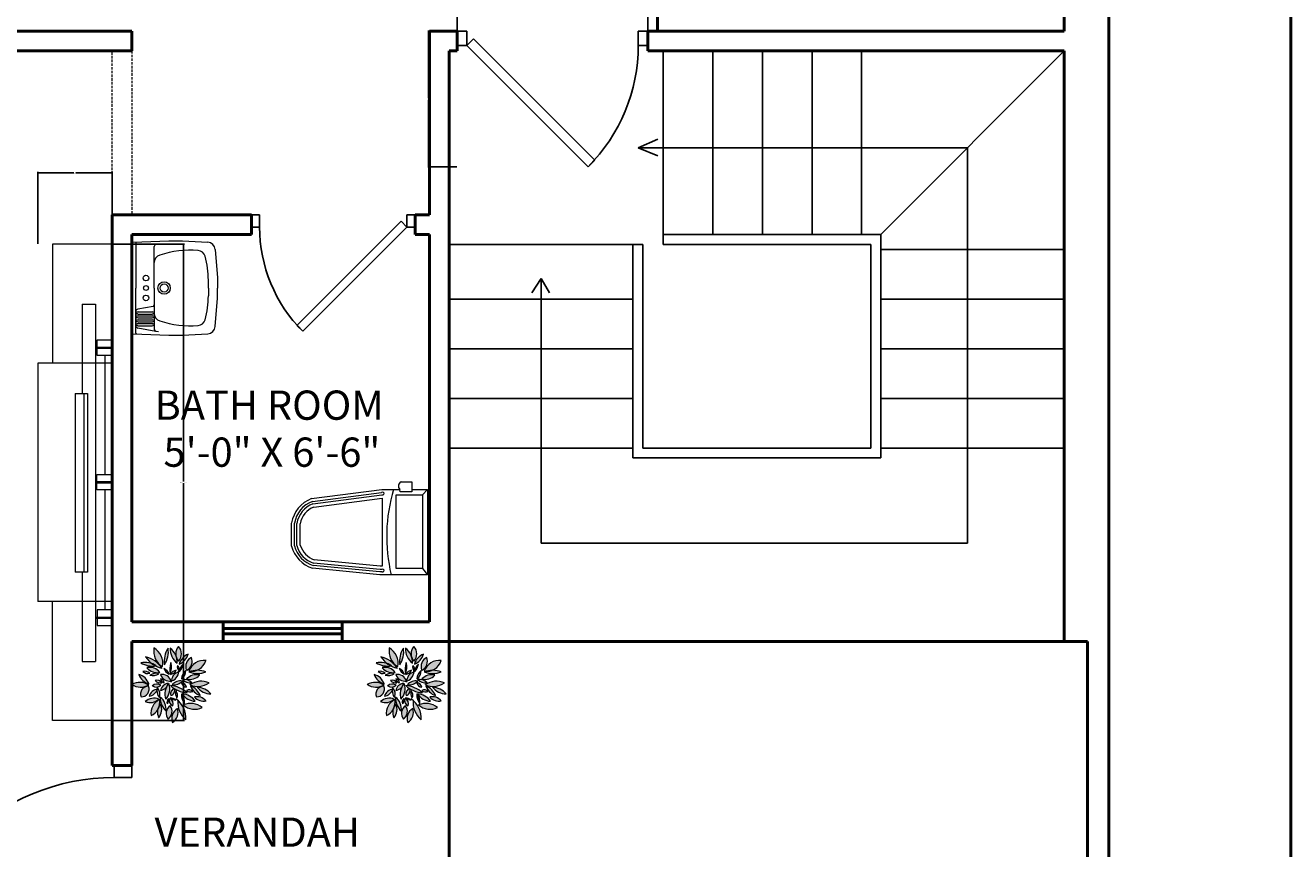
# Model space of a CAD drawing. Units: inches. Extents: x 64 to 1167, y 117 to 939.
# Tile 4 of 56: x 258 to 513, y 272 to 438. Entities that reach past the tile are written whole.
import ezdxf

# ---------------------------------------------------------------- set-up
doc = ezdxf.new("R2010")
doc.units = ezdxf.units.IN
doc.header["$MEASUREMENT"] = 0
doc.linetypes.add('DASHED', pattern=[0.75, 0.5, -0.25])
for name, color, linetype, lineweight in [('A-ANNO-DIMS', 2, 'Continuous', 18), ('A-ANNO-TEXT', 7, 'Continuous', 25), ('A-ANNO-TTLB', 7, 'Continuous', 50), ('A-DOOR', 4, 'Continuous', 25), ('A-FLOR-FIXT', 8, 'Continuous', 18), ('A-FLOR-OVHD', 8, 'DASHED', 18), ('A-FLOR-STRS', 3, 'Continuous', 25), ('A-FURN', 8, 'Continuous', 18), ('A-WALL', 7, 'Continuous', 50)]:
    doc.layers.add(name, color=color, linetype=linetype, lineweight=lineweight)
doc.styles.get("Standard").update_dxf_attribs({"font": 'arial.ttf'})
doc.dimstyles.get("Standard").update_dxf_attribs({"dimtxt": 0.18, "dimasz": 0.18, "dimexe": 0.18, "dimexo": 0.0625, "dimgap": 0.09, "dimtad": 0, "dimtih": 1, "dimtoh": 1, "dimdec": 4, "dimzin": 0, "dimdsep": 46, "dimtxsty": 'Standard', "dimcen": 0.09, "dimadec": 0, "dimazin": 0, "dimtfac": 1, "dimtdec": 4, "dimtofl": 0, "dimtmove": 0, "dimatfit": 3, "dimfxl": 1, "dimtolj": 1, "dimtzin": 0, "dimarcsym": 0})

# ---------------------------------------------------------------- blocks, each defined once
blk = doc.blocks.new('A$C68901CC0')
for p, q in [((10.95, 26.62), (12.35, 28.01)), ((12.35, 28.01), (37.4, 2.95)), ((36.01, 1.56), (10.95, 26.62)), ((0, 2.95), (0, 0)), ((1.97, 2.95), (0, 2.95)), ((1.97, 0), (1.97, 2.95)), ((37.4, 2.95), (36.01, 1.56)), ((37.4, 2.95), (37.4, 0)), ((39.37, 2.95), (37.4, 2.95)), ((39.37, 0), (39.37, 2.95)), ((0, 0), (1.97, 0)), ((37.4, 0), (39.37, 0))]:
    blk.add_line(p, q)
blk.add_arc((37.4, 2.95), 35.43, 135, 180)
blk = doc.blocks.new("CONSOLE 8'x1'3")
for p, q in [((-48, 0), (48, 0)), ((48, 0), (48, -12)), ((-48, 0), (-48, -12)), ((-24, 0), (-24, -15)), ((24, 0), (24, -15)), ((-48, -12), (-24, -12)), ((48, -12), (24, -12)), ((-24, -15), (24, -15))]:
    blk.add_line(p, q)
blk = doc.blocks.new('A$C2B992F40')
for p, q in [((39.2, 615.2), (39.2, 696.2)), ((39.2, 696.2), (475.7, 696.2)), ((66.8, 669.7), (39.2, 696.2)), ((66.8, 534.6), (66.8, 669.7)), ((66.8, 669.7), (444.2, 669.7)), ((444.2, 669.7), (475.7, 696.2)), ((444.2, 669.7), (444.2, 534.6)), ((475.7, 696.2), (475.7, 509.8)), ((0, 561.3), (0, 615.2)), ((0, 615.2), (51.5, 615.2)), ((51.5, 615.2), (51.5, 556.4)), ((51.5, 556.4), (39.2, 553.9)), ((39.2, 522.1), (39.2, 553.9)), ((40.1, 461.2), (39.2, 522.1)), ((444.2, 534.6), (66.8, 534.6)), ((86.6, 102.5), (40.1, 461.2)), ((101, 106.1), (55, 460.6)), ((112.5, 109), (66.6, 462.1)), ((84.2, 464.4), (431.5, 464.4)), ((129.7, 113.4), (84.2, 464.4)), ((431.5, 454), (399.6, 116.2)), ((431.5, 464.4), (431.5, 454)), ((449.2, 464.4), (449.2, 453.2)), ((461, 464.4), (461, 452.6)), ((475.7, 509.8), (475.7, 451.9)), ((449.2, 453.2), (417, 112.5)), ((461, 452.6), (428.6, 110.1)), ((475.7, 451.9), (443.1, 107.2)), ((330.1, 0), (211.3, 0)), ((328.2, 14.7), (212.5, 14.7)), ((326.7, 26.5), (213.4, 26.5)), ((324.2, 44.1), (215, 44.1))]:
    blk.add_line(p, q)
for centre, radius, start, end in [((22.2, 571.4), 24.4, 204.49972, 314.26101), ((280.3, 1327.8), 841, 253.34642, 283.43557), ((60.2, 466.1), 7.56, 328.52932, 226.26991), ((454.4, 466.1), 7.56, 328.52932, 226.26991), ((235.9, 157), 158.9, 200.05507, 261.07522), ((235.9, 157), 144.2, 200.68762, 260.63012), ((235.9, 157), 132.4, 201.26818, 260.22173), ((235.9, 157), 114.8, 202.30203, 259.4948), ((291.5, 153.8), 114.4, 286.5809, 340.81554), ((291.5, 153.8), 132.1, 285.42576, 341.7737), ((291.5, 153.8), 143.8, 284.77755, 342.31156), ((291.5, 153.8), 158.5, 284.07165, 342.89742)]:
    blk.add_arc(centre, radius, start, end)
blk = doc.blocks.new("FLAT TV 6'")
for p, q in [((2564.73, 835.73), (2564.73, 838.99)), ((2564.97, 835.73), (2564.97, 838.99)), ((2566.41, 837.49), (2590.37, 837.49)), ((2591.81, 835.67), (2591.81, 838.93)), ((2592.05, 835.67), (2592.05, 838.93)), ((2593.49, 837.49), (2617.69, 837.49)), ((2619.13, 835.73), (2619.13, 838.99)), ((2619.37, 835.73), (2619.37, 838.99)), ((2556.05, 835.67), (2628.05, 835.67)), ((2556.05, 832.92), (2556.05, 835.67)), ((2628.05, 832.92), (2628.05, 835.67)), ((2556.05, 832.92), (2574.05, 832.92)), ((2574.05, 831.54), (2574.05, 834.04)), ((2574.05, 834.04), (2610.05, 834.04)), ((2574.05, 833.29), (2610.05, 833.29)), ((2610.05, 834.04), (2610.05, 831.54)), ((2610.05, 832.92), (2628.05, 832.92)), ((2574.05, 831.54), (2610.05, 831.54))]:
    blk.add_line(p, q)
for points in [[(2563.29, 838.99), (2566.41, 838.99), (2566.41, 835.99), (2563.29, 835.99)], [(2590.37, 838.93), (2593.49, 838.93), (2593.49, 835.93), (2590.37, 835.93)], [(2620.82, 838.99), (2617.69, 838.99), (2617.69, 835.99), (2620.82, 835.99)]]:
    blk.add_lwpolyline(points, close=True)
blk = doc.blocks.new('A$C172C5132')
at = {"linetype": 'ByBlock'}
h = blk.add_hatch(color=256, dxfattribs=at)
h.set_gradient(color1=(15, 138, 17), color2=(46, 92, 10), tint=1, name='HEMISPHERICAL')
h.paths.add_polyline_path([(0.0849, 0.0409, 0.236282), (0.1, 0.0045, 0.236282)])
h.paths.add_polyline_path([(0.0951, 0.0322, 0.290628), (0.1303, 0.0274, 0.290628)])
h.paths.add_polyline_path([(0.0751, 0, 0.364082), (0.0843, 0.0256, 0.364082)])
h.paths.add_polyline_path([(0.0708, 0.0309, 0.428936), (0.0669, 0.0061, 0.428936)])
h.paths.add_polyline_path([(0.0526, 0.0469, 0.243055), (0.0634, 0.0209, 0.243055)])
h.paths.add_polyline_path([(0.0509, 0.0311, -0.075692), (0.0478, 0.0235, 0.164666), (0.0495, 0.0087, 0.298636), (0.053, 0.0339, 0.03785)])
h.paths.add_polyline_path([(0.0356, 0.0126, 0.152567), (0.0478, 0.0235, -0.089408), (0.0509, 0.0311, 0.1023), (0.0513, 0.0422, 0.341288)])
h.paths.add_polyline_path([(0.0248, 0.0387, 0.299202), (0.0498, 0.0428, 0.299202)])
h.paths.add_polyline_path([(0.0475, 0.0637, 0.031182), (0.0468, 0.0616, -0.006707), (0.0473, 0.0617), (0.0473, 0.0617), (0.0473, 0.0617, -0.03138), (0.0464, 0.0594, 0.214704), (0.0508, 0.0461, 0.282795)])
h.paths.add_polyline_path([(0.0643, 0.0658, 0.211659), (0.0625, 0.043, 0.281051), (0.0686, 0.0717, 0.038772), (0.0659, 0.0683, -0.044717)])
h.paths.add_polyline_path([(0.053, 0.0591, 0.203733), (0.0643, 0.0658, -0.026656), (0.0659, 0.0683, 0.062829), (0.0673, 0.0723, 0.318582)])
h.paths.add_polyline_path([(0.0695, 0.0439, 0.403257), (0.076, 0.0304, 0.403257)])
h.paths.add_polyline_path([(0.0652, 0.0343, 0.302607), (0.0678, 0.0439, 0.302607)])
h.paths.add_polyline_path([(0.0708, 0.0452, 0.20419), (0.0817, 0.0413, 0.20419)])
h.paths.add_polyline_path([(0.0817, 0.0582, 0.262138), (0.0834, 0.0452, 0.262138)])
h.paths.add_polyline_path([(0.0721, 0.05, 0.44636), (0.0791, 0.0622, 0.44636)])
h.paths.add_polyline_path([(0.0934, 0.0526, 0.247085), (0.1173, 0.0391, 0.247085)])
h.paths.add_polyline_path([(0.0712, 0.0682, 0.171467), (0.1021, 0.0548, 0.171467)])
h.paths.add_polyline_path([(0.0747, 0.07, 0.259278), (0.0934, 0.0765, 0.259278)])
h.paths.add_polyline_path([(0.0917, 0.073, 0.365639), (0.1012, 0.0652, 0.365639)])
h.paths.add_polyline_path([(0.0934, 0.0795, 0.243415), (0.1108, 0.0735, 0.243415)])
h.paths.add_polyline_path([(0.1012, 0.0591, 0.307451), (0.1129, 0.0574, 0.307451)])
h.paths.add_polyline_path([(0.1086, 0.0674, 0.209633), (0.1264, 0.0496, 0.209633)])
h.paths.add_polyline_path([(0.1208, 0.0652, 0.21311), (0.1464, 0.0526, 0.21311)])
h.paths.add_polyline_path([(0.116, 0.0469, 0.265719), (0.1373, 0.04, 0.265719)])
h.paths.add_polyline_path([(0.1012, 0.0804, 0.271534), (0.1255, 0.0874, 0.271534)])
h.paths.add_polyline_path([(0.1204, 0.0965, -0.10541), (0.1084, 0.0945, 0.018052), (0.1055, 0.0935, 0.194763), (0.1373, 0.0935, 0.102488)])
h.paths.add_polyline_path([(0.1055, 0.0948, 0.024701), (0.1084, 0.0945, -0.072299), (0.1204, 0.0965, 0.220444), (0.1373, 0.1143, 0.361284)])
h.paths.add_polyline_path([(0.0921, 0.0808, 0.244188), (0.0999, 0.0961, 0.244188)])
h.paths.add_polyline_path([(0.0873, 0.1078, 0.236039), (0.1042, 0.1265, 0.236039)])
h.paths.add_polyline_path([(0.0843, 0.1056, 0.271887), (0.0875, 0.0951, 0.271887)])
h.paths.add_polyline_path([(0.073, 0.0766, -0.001193), (0.073, 0.0765, 0.325344), (0.0864, 0.0931, 0.324468)])
h.paths.add_polyline_path([(0.0713, 0.0905, 0.143951), (0.0721, 0.1108, 0.143951)])
h.paths.add_polyline_path([(0.0591, 0.1, 0.207976), (0.0691, 0.0891, 0.207976)])
h.paths.add_polyline_path([(0.0604, 0.1065, 0.190107), (0.0669, 0.1374, 0.190107)])
h.paths.add_polyline_path([(0.0708, 0.1374, 0.252904), (0.0838, 0.1095, 0.067921), (0.0831, 0.1182, -0.074796), (0.0813, 0.124, 0.134159)])
h.paths.add_polyline_path([(0.0813, 0.124, -0.046564), (0.0831, 0.1182, 0.072445), (0.0864, 0.1134, 0.391074), (0.0864, 0.1408, 0.229731)])
h = blk.add_hatch(color=256, dxfattribs=at)
h.set_gradient(color1=(12, 110, 14), color2=(39, 78, 9), tint=1, name='HEMISPHERICAL')
h.paths.add_polyline_path([(0.0278, 0.1013, 0.287265), (0.0517, 0.0926, 0.287265)])
h.paths.add_polyline_path([(0.0334, 0.0874, 0.245454), (0.05, 0.09, 0.245454)])
h.paths.add_polyline_path([(0.053, 0.0887, 0.362884), (0.0729, 0.0765, -0.000877), (0.073, 0.0766, 0.362272)])
h.paths.add_polyline_path([(0.053, 0.0808, 0.33327), (0.0599, 0.073, 0.33327)])
h.paths.add_polyline_path([(0.043, 0.0778, 0.302945), (0.0552, 0.0735, 0.302945)])
h.paths.add_polyline_path([(0.0378, 0.0674, 0.378763), (0.0534, 0.0687, 0.378763)])
h.paths.add_polyline_path([(0.0317, 0.0482, 0.247698), (0.0464, 0.0594, -0.032946), (0.0468, 0.0616, 0.274039)])
h.paths.add_polyline_path([(0.0169, 0.0474, 0.549808), (0.0308, 0.0669, 0.549808)])
h.paths.add_polyline_path([(0, 0.0704, 0.297781), (0.0304, 0.069, 0.297781)])
h.paths.add_polyline_path([(0.013, 0.0887, 0.248111), (0.0313, 0.0713, 0.248111)])
h.paths.add_polyline_path([(0.0204, 0.0943, 0.290415), (0.033, 0.0908, 0.290415)])
h.paths.add_polyline_path([(0.0165, 0.1104, 0.175406), (0.0437, 0.1045, -0.037323), (0.0372, 0.1086, 0.129374)])
h.paths.add_polyline_path([(0.0252, 0.1213, 0.085647), (0.0372, 0.1086, -0.054384), (0.0452, 0.1048), (0.0452, 0.1048, -0.009351), (0.0437, 0.1045, 0.060507), (0.0552, 0.1), (0.0556, 0.1006, 0.185254)])
h.paths.add_polyline_path([(0.0408, 0.1378, 0.313266), (0.0566, 0.1033), (0.0567, 0.1033, 0.313266)])
h.paths.add_polyline_path([(0.0712, 0.0891), (0.0716, 0.0886, 0.230232), (0.0821, 0.0965, 0.230232)])
h.paths.add_polyline_path([(0.0877, 0.0943), (0.0881, 0.0941, 0.179345), (0.0947, 0.1078, 0.179345)])
h.paths.add_polyline_path([(0.1008, 0.0968), (0.1016, 0.0965, 0.378282), (0.1103, 0.1204, 0.378282)])
h = blk.add_hatch(color=256, dxfattribs=at)
h.set_gradient(color1=(12, 110, 14), color2=(39, 78, 9), tint=1, name='HEMISPHERICAL')
h.paths.add_polyline_path([(0.1077, 0.0699), (0.1077, 0.0695, 0.262244), (0.1429, 0.073, 0.262244)])
h = blk.add_hatch(color=256)
h.set_gradient(color1=(12, 110, 14), color2=(39, 78, 9), tint=1, name='HEMISPHERICAL')
h.paths.add_polyline_path([(0.0925, 0.0526), (0.092, 0.0525, 0.192472), (0.0973, 0.0343, 0.192472)])
for p, q in [((0.0552, 0.1), (0.0556, 0.1006)), ((0.0566, 0.1033), (0.0567, 0.1033)), ((0.0881, 0.0941), (0.0877, 0.0943)), ((0.1016, 0.0965), (0.1008, 0.0968)), ((0.0716, 0.0886), (0.0712, 0.0891)), ((0.0925, 0.0526), (0.092, 0.0525)), ((0.1077, 0.0695), (0.1077, 0.0699))]:
    blk.add_line(p, q, dxfattribs=at)
for centre, radius, start, end in [((0.1013, 0.1271), 0.0202, 137.2816, 222.7184), ((0.0716, 0.1271), 0.0202, 317.2816, 42.7184), ((0.0135, 0.0713), 0.0513, 34.8518, 76.8329), ((0.0679, 0.1498), 0.0513, 213.7346, 255.7157), ((0.0736, 0.1319), 0.0333, 169.7437, 239.3198), ((0.024, 0.1091), 0.0333, 349.9797, 59.5558), ((0.1028, 0.1137), 0.043, 146.5506, 189.6063), ((0.0245, 0.1302), 0.043, 326.5506, 9.6063), ((0.1031, 0.1355), 0.0323, 176.7146, 233.4855), ((0.0516, 0.1114), 0.0323, 356.7146, 53.4855), ((0.1145, 0.1002), 0.0282, 111.2499, 164.3738), ((0.0771, 0.1341), 0.0282, 291.2499, 344.3738), ((0.1189, 0.1032), 0.0192, 116.5049, 199.3878), ((0.0924, 0.1134), 0.0192, 298.5878, 21.4707), ((0.0235, 0.0702), 0.0408, 57.8807, 99.8189), ((0.0382, 0.145), 0.0408, 237.8807, 279.8189), ((0.024, 0.0827), 0.0122, 42.1798, 106.9561), ((0.0295, 0.1025), 0.0122, 222.1798, 286.9561), ((0.0328, 0.0779), 0.024, 37.9495, 102.0596), ((0.0467, 0.116), 0.024, 217.9495, 282.0596), ((0.0516, 0.083), 0.0185, 19.0975, 66.0922), ((0.0766, 0.106), 0.0185, 199.0975, 246.0922), ((0.1064, 0.0993), 0.0362, 161.3279, 196.3785), ((0.037, 0.102), 0.0362, 339.0434, 14.094), ((0.0682, 0.094), 0.0182, 278.3256, 1.7816), ((0.0843, 0.0816), 0.015, 98.3028, 150.1644), ((0.0688, 0.1034), 0.015, 280.7404, 332.602), ((0.0949, 0.1031), 0.0109, 166.6712, 231.5788), ((0.0769, 0.0976), 0.0109, 342.6051, 47.5126), ((0.1094, 0.0917), 0.0218, 132.3809, 173.0513), ((0.073, 0.1098), 0.0218, 313.9894, 354.6599), ((0.0813, 0.096), 0.0186, 305.3547, 0.2444), ((0.1106, 0.0809), 0.0186, 125.3547, 180.2444), ((0.1332, 0.0855), 0.0291, 81.9405, 161.3964), ((0.1096, 0.1236), 0.0291, 261.9405, 341.3964), ((0.1214, 0.0543), 0.0422, 67.9577, 112.0423), ((0.0141, 0.0464), 0.0278, 52.0955, 120.5238), ((0.0163, 0.093), 0.0278, 234.1936, 302.622), ((0.0386, 0.0972), 0.027, 198.5093, 254.2466), ((0.0057, 0.0627), 0.027, 18.5093, 74.2466), ((0.0442, 0.0729), 0.018, 71.397, 126.5601), ((0.0392, 0.1045), 0.018, 251.397, 306.5601), ((0.0463, 0.0592), 0.0118, 53.2772, 136.2565), ((0.0458, 0.0665), 0.0116, 36.6262, 104.0418), ((0.0523, 0.0847), 0.0116, 216.6262, 284.0418), ((0.0557, 0.0706), 0.0182, 18.7265, 98.5819), ((0.0703, 0.0945), 0.0182, 198.7265, 278.5819), ((0.0512, 0.0723), 0.00872, 4.751, 78.4779), ((0.0617, 0.0816), 0.00872, 184.751, 258.4779), ((0.0508, 0.0758), 0.0168, 277.3883, 349.0703), ((0.0694, 0.0556), 0.0168, 96.3902, 168.0722), ((0.0891, 0.0524), 0.0281, 136.6356, 199.4278), ((0.0421, 0.0624), 0.0281, 316.6356, 19.4278), ((0.0911, 0.0756), 0.0182, 100.5964, 184.0524), ((0.0899, 0.0564), 0.0204, 80.1717, 138.3136), ((0.0782, 0.09), 0.0204, 260.1717, 318.3136), ((0.0918, 0.0634), 0.00957, 10.523, 90.8605), ((0.1011, 0.0748), 0.00957, 190.523, 270.8605), ((0.0962, 0.0597), 0.02, 43.3367, 98.0592), ((0.108, 0.0933), 0.02, 223.3367, 278.0592), ((0.1193, 0.0631), 0.025, 75.5726, 136.3385), ((0.1074, 0.1046), 0.025, 255.5726, 316.3385), ((0.1214, 0.1326), 0.0422, 247.9577, 292.0423), ((0.1281, 0.0402), 0.036, 65.6693, 124.4476), ((0.1222, 0.1025), 0.036, 246.2552, 305.0335), ((0.0301, 0.0527), 0.0142, 86.9965, 202.2058), ((0.0177, 0.0616), 0.0142, 266.9965, 22.2058), ((0.0285, 0.0678), 0.0198, 279.3324, 342.1699), ((0.0506, 0.0422), 0.0198, 99.3324, 162.1699), ((0.0449, 0.0769), 0.0118, 233.2772, 316.2565), ((0.0634, 0.0576), 0.0171, 157.7122, 222.4235), ((0.0348, 0.0521), 0.0171, 339.261, 43.9723), ((0.0832, 0.0444), 0.0308, 175.2839, 229.9285), ((0.0327, 0.0234), 0.0308, 355.2839, 49.9285), ((0.1057, 0.1051), 0.0505, 226.9394, 265.8583), ((0.0676, 0.0179), 0.0505, 46.9394, 85.8583), ((0.081, 0.053), 0.00941, 102.1635, 198.3798), ((0.0701, 0.0592), 0.00941, 282.1635, 18.3798), ((0.0941, 0.0533), 0.0134, 158.2119, 216.9673), ((0.0709, 0.0502), 0.0134, 338.2119, 36.9673), ((0.1173, 0.05), 0.0254, 174.4977, 218.0761), ((0.0721, 0.0375), 0.0254, 352.8778, 36.4562), ((0.1181, 0.0686), 0.0294, 212.8184, 268.3343), ((0.0925, 0.0232), 0.0294, 32.8184, 88.3343), ((0.1058, 0.0496), 0.0106, 47.3873, 115.7476), ((0.1084, 0.0669), 0.0106, 227.3873, 295.7476), ((0.0972, 0.0382), 0.0314, 21.3015, 68.66), ((0.1378, 0.0788), 0.0314, 201.3015, 248.66), ((0.1205, 0.0249), 0.0226, 42.1437, 101.6667), ((0.1327, 0.0621), 0.0226, 222.1437, 281.6667), ((0.1195, 0.0302), 0.035, 39.7488, 87.8702), ((0.1477, 0.0876), 0.035, 219.7488, 267.8702), ((0.0404, 0.0217), 0.0231, 65.4893, 132.7752), ((0.0341, 0.0598), 0.0231, 246.1459, 313.4318), ((0.0626, 0.0173), 0.0273, 114.4303, 189.807), ((0.0243, 0.0375), 0.0273, 294.4303, 9.807), ((0.0705, 0.0186), 0.0232, 138.8969, 205.4069), ((0.032, 0.0239), 0.0232, 318.8969, 25.4069), ((0.0806, 0.0166), 0.0173, 124.6008, 217.4658), ((0.0736, 0.0372), 0.00894, 131.0823, 198.427), ((0.0593, 0.0411), 0.00894, 311.0823, 18.427), ((0.0571, 0.0203), 0.0173, 304.6008, 37.4658), ((0.0798, 0.0405), 0.0108, 161.8817, 249.7301), ((0.0658, 0.0338), 0.0108, 341.8817, 69.7301), ((0.0808, 0.056), 0.0147, 227.1077, 273.2701), ((0.0716, 0.0305), 0.0147, 47.1077, 93.2701), ((0.095, 0.0074), 0.0212, 120.4086, 200.4312), ((0.0644, 0.0183), 0.0212, 300.4086, 20.4312), ((0.056, 0.0075), 0.0441, 356.0096, 54.5768), ((0.1289, 0.0379), 0.0441, 176.0096, 229.186), ((0.109, 0.0021), 0.0331, 49.8506, 114.6719), ((0.1165, 0.0575), 0.0331, 229.8506, 294.6719)]:
    blk.add_arc(centre, radius, start, end, dxfattribs=at)
blk = doc.blocks.new('A$C056A4ABE')
at = {"ltscale": 20}
for p, q in [((0.0065, 0.4339), (0, 0.2479)), ((0.0098, 0.4178), (0.2406, 0.4178)), ((0.2406, 0.4378), (0.0105, 0.4378)), ((0.0188, 0.315), (0.0351, 0.4075)), ((0.0472, 0.4063), (0.0472, 0.3333)), ((0.1205, 0.4178), (0.0475, 0.4178)), ((0.11, 0.4178), (0.0579, 0.4178)), ((0.0582, 0.4063), (0.0582, 0.3333)), ((0.0672, 0.4063), (0.0672, 0.3333)), ((0.0782, 0.4063), (0.0782, 0.3333)), ((0.0872, 0.4063), (0.0872, 0.3333)), ((0.0982, 0.4063), (0.0982, 0.3333)), ((0.1072, 0.4063), (0.1072, 0.3333)), ((0.1182, 0.4063), (0.1182, 0.3333)), ((0.1465, 0.3295), (0.1328, 0.4075)), ((0.2406, 0.4378), (0.4708, 0.4378)), ((0.4715, 0.4178), (0.2406, 0.4178)), ((0.4748, 0.4339), (0.4813, 0.2479)), ((0.0164, 0.3013), (0.0188, 0.315)), ((0.2406, 0.3233), (0.0287, 0.3233)), ((0.2406, 0.3233), (0.1468, 0.3233)), ((0.2406, 0.3233), (0.3344, 0.3233)), ((0.2406, 0.3233), (0.4526, 0.3233)), ((0.4648, 0.3013), (0.4624, 0.315)), ((0, 0.2479), (0, 0.1789)), ((0.4813, 0.2479), (0.4813, 0.1789)), ((0, 0.1789), (0.0068, 0.0492)), ((0.4813, 0.1789), (0.4745, 0.0492)), ((0.0436, 0.0114), (0.1881, 0)), ((0.1881, 0), (0.2406, 0)), ((0.2406, 0.0463), (0.2011, 0.0463)), ((0.2406, 0.0463), (0.2802, 0.0463)), ((0.2932, 0), (0.2406, 0)), ((0.4377, 0.0114), (0.2932, 0))]:
    blk.add_line(p, q, dxfattribs=at)
for centre, radius in [((0.1896, 0.3658), 0.0143), ((0.2406, 0.3658), 0.0125), ((0.2916, 0.3658), 0.0143), ((0.2406, 0.2728), 0.0315), ((0.2406, 0.2728), 0.0205)]:
    blk.add_circle(centre, radius, dxfattribs=at)
for centre, radius, start, end in [((0.0098, 0.4138), 0.004, 90, 178), ((0.0105, 0.4338), 0.004, 90, 178), ((0.0475, 0.4053), 0.0125, 90, 170), ((0.0527, 0.4063), 0.0055, 0, 172.14641), ((0.0727, 0.4063), 0.0055, 0, 180), ((0.0927, 0.4063), 0.0055, 0, 180), ((0.1127, 0.4063), 0.0055, 0, 180), ((0.1205, 0.4053), 0.0125, 10, 90), ((0.4708, 0.4338), 0.004, 2, 90), ((0.4715, 0.4138), 0.004, 2, 90), ((0.0527, 0.3333), 0.0055, 180, 0), ((0.0727, 0.3333), 0.0055, 180, 0), ((0.0927, 0.3333), 0.0055, 180, 0), ((0.1127, 0.3333), 0.0055, 180, 0), ((0.1539, 0.3308), 0.0075, 190, 270), ((0.0287, 0.3133), 0.01, 90, 170), ((0.5633, 0.1363), 0.516, 162.04923, 184.18169), ((0.1106, 0.2833), 0.04, 90, 162.51071), ((0.3706, 0.2833), 0.04, 17.48929, 90), ((-0.0821, 0.1363), 0.516, 355.81831, 17.95077), ((0.4526, 0.3133), 0.01, 10, 90), ((0.0886, 0.1016), 0.04, 184.18128, 254.50873), ((0.3926, 0.1016), 0.04, 285.49127, 355.81872), ((0.0467, 0.0512), 0.04, 183, 265.5), ((0.2011, 0.5073), 0.461, 254.50873, 270), ((0.2802, 0.5073), 0.461, 270, 285.49127), ((0.4345, 0.0512), 0.04, 274.5, 357)]:
    blk.add_arc(centre, radius, start, end, dxfattribs=at)
blk = doc.blocks.new('*D62')
at = {"layer": 'A-ANNO-DIMS', "color": 0, "lineweight": -2, "transparency": 16777216}
for p, q in [((344.69, 437.26), (344.69, 443.15)), ((344.87, 442.97), (363.29, 442.97)), ((382.96, 442.97), (364.54, 442.97)), ((383.14, 437.26), (383.14, 443.15))]:
    blk.add_line(p, q, dxfattribs=at)
for points in [[(344.87, 443), (344.87, 442.94), (344.69, 442.97)], [(382.96, 443), (382.96, 442.94), (383.14, 442.97)]]:
    blk.add_solid(points, dxfattribs=at)
at = {"layer": 'Defpoints', "color": 0, "lineweight": -2, "transparency": 16777216}
for p in [(344.69, 442.97), (344.69, 437.2), (383.14, 437.2)]:
    blk.add_point(p, dxfattribs=at)
at = {"layer": 'A-ANNO-DIMS', "color": 0, "transparency": 16777216, "insert": (363.91, 442.97), "char_height": 0.18, "attachment_point": 5}
blk.add_mtext('\\A1;DOOR 38', dxfattribs=at)
blk = doc.blocks.new('*D63')
at = {"layer": 'A-ANNO-DIMS', "color": 0, "lineweight": -2, "transparency": 16777216}
for p, q in [((344.63, 437.2), (338.75, 437.2)), ((338.93, 437.02), (338.93, 423.71)), ((338.93, 410.03), (338.93, 423.35)), ((344.63, 409.85), (338.75, 409.85))]:
    blk.add_line(p, q, dxfattribs=at)
for points in [[(338.9, 437.02), (338.96, 437.02), (338.93, 437.2)], [(338.9, 410.03), (338.96, 410.03), (338.93, 409.85)]]:
    blk.add_solid(points, dxfattribs=at)
at = {"layer": 'Defpoints', "color": 0, "lineweight": -2, "transparency": 16777216}
for p in [(344.69, 437.2), (338.93, 409.85), (344.69, 409.85)]:
    blk.add_point(p, dxfattribs=at)
at = {"layer": 'A-ANNO-DIMS', "color": 0, "transparency": 16777216, "insert": (338.93, 423.53), "char_height": 0.18, "attachment_point": 5}
blk.add_mtext('\\A1;27', dxfattribs=at)
blk = doc.blocks.new('*D84')
at = {"layer": 'A-ANNO-DIMS', "color": 0, "lineweight": -2, "transparency": 16777216}
for p, q in [((275.17, 394.27), (289.69, 394.27)), ((289.51, 394.09), (289.51, 346.46)), ((289.51, 298.45), (289.51, 346.09)), ((275.17, 298.27), (289.69, 298.27))]:
    blk.add_line(p, q, dxfattribs=at)
for points in [[(289.48, 394.09), (289.54, 394.09), (289.51, 394.27)], [(289.48, 298.45), (289.54, 298.45), (289.51, 298.27)]]:
    blk.add_solid(points, dxfattribs=at)
at = {"layer": 'Defpoints', "color": 0, "lineweight": -2, "transparency": 16777216}
for p in [(275.11, 394.27), (275.11, 298.27), (289.51, 298.27)]:
    blk.add_point(p, dxfattribs=at)
at = {"layer": 'A-ANNO-DIMS', "color": 0, "transparency": 16777216, "insert": (289.51, 346.27), "char_height": 0.18, "attachment_point": 5}
blk.add_mtext('\\A1;CONSOLE 96', dxfattribs=at)
blk = doc.blocks.new('*D85')
at = {"layer": 'A-ANNO-DIMS', "color": 0, "lineweight": -2, "transparency": 16777216}
for p, q in [((260.11, 394.34), (260.11, 408.85)), ((260.29, 408.67), (267.4, 408.67)), ((274.93, 408.67), (267.82, 408.67)), ((275.11, 394.34), (275.11, 408.85))]:
    blk.add_line(p, q, dxfattribs=at)
for points in [[(260.29, 408.7), (260.29, 408.64), (260.11, 408.67)], [(274.93, 408.7), (274.93, 408.64), (275.11, 408.67)]]:
    blk.add_solid(points, dxfattribs=at)
at = {"layer": 'Defpoints', "color": 0, "lineweight": -2, "transparency": 16777216}
for p in [(275.11, 408.67), (260.11, 394.27), (275.11, 394.27)]:
    blk.add_point(p, dxfattribs=at)
at = {"layer": 'A-ANNO-DIMS', "color": 0, "transparency": 16777216, "insert": (267.61, 408.67), "char_height": 0.18, "attachment_point": 5}
blk.add_mtext('\\A1;15', dxfattribs=at)

msp = doc.modelspace()

# ---------------------------------------------------------------- linework, layer by layer
at = {"layer": 'A-ANNO-TTLB'}
msp.add_lwpolyline([(64.31, 939.22), (512.77, 939.22), (512.77, 116.55), (64.31, 116.55)], close=True, dxfattribs=at)
at = {"layer": 'A-FLOR-OVHD'}
for p, q in [((275.11, 400.2), (275.11, 433.2)), ((279.11, 433.2), (279.11, 400.2))]:
    msp.add_line(p, q, dxfattribs=at)
at = {"layer": 'A-FLOR-STRS'}
for p, q in [((386.25, 433.2), (386.25, 394.2)), ((396.25, 433.2), (396.25, 396.2)), ((406.25, 433.2), (406.25, 396.2)), ((416.25, 433.2), (416.25, 396.2)), ((426.25, 433.2), (426.25, 396.2)), ((430.11, 396.2), (467.11, 433.2)), ((381.2, 413.7), (385.18, 415.45)), ((381.2, 413.7), (447.61, 413.7)), ((381.2, 413.7), (385.14, 412.08)), ((447.61, 413.7), (447.61, 334.04)), ((430.11, 396.2), (386.25, 396.2)), ((430.11, 396.2), (430.11, 351.2)), ((382.11, 394.2), (343.11, 394.2)), ((380.11, 394.2), (380.11, 351.2)), ((382.11, 394.2), (382.11, 353.2)), ((428.11, 394.2), (386.25, 394.2)), ((428.11, 394.2), (428.11, 353.2)), ((430.11, 393.2), (467.11, 393.2)), ((361.61, 387.35), (359.74, 384.47)), ((361.61, 334.04), (361.61, 387.35)), ((361.61, 387.35), (363.3, 384.47)), ((343.11, 383.2), (380.11, 383.2)), ((430.11, 383.2), (467.11, 383.2)), ((343.11, 373.2), (380.11, 373.2)), ((430.11, 373.2), (467.11, 373.2)), ((343.11, 363.2), (380.11, 363.2)), ((430.11, 363.2), (467.11, 363.2)), ((343.11, 353.2), (380.11, 353.2)), ((382.11, 353.2), (428.11, 353.2)), ((430.11, 353.2), (467.11, 353.2)), ((380.11, 351.2), (430.11, 351.2)), ((447.61, 334.04), (361.61, 334.04))]:
    msp.add_line(p, q, dxfattribs=at)
at = {"layer": 'A-WALL'}
for p, q in [((476.11, 863.2), (476.11, 155.2)), ((467.11, 581.2), (467.11, 437.2)), ((385.11, 461.2), (385.11, 437.2)), ((279.11, 437.2), (255.11, 437.2)), ((279.11, 437.2), (279.11, 433.2)), ((339.11, 437.2), (339.11, 400.2)), ((344.69, 437.2), (339.11, 437.2)), ((344.69, 437.2), (344.69, 433.2)), ((385.11, 437.2), (383.14, 437.2)), ((383.14, 437.2), (383.14, 433.2)), ((467.11, 437.2), (385.11, 437.2)), ((279.11, 433.2), (131.11, 433.2)), ((343.11, 433.2), (343.11, 314.2)), ((344.69, 433.2), (343.11, 433.2)), ((467.11, 433.2), (383.14, 433.2)), ((467.11, 433.2), (467.11, 314.2)), ((275.11, 400.2), (275.11, 289.2)), ((303.2, 400.2), (275.11, 400.2)), ((303.2, 396.2), (303.2, 400.2)), ((339.11, 400.2), (336.19, 400.2)), ((336.19, 396.2), (336.19, 400.2)), ((279.11, 396.2), (279.11, 318.2)), ((303.2, 396.2), (279.11, 396.2)), ((339.11, 396.2), (336.19, 396.2)), ((339.11, 396.2), (339.11, 318.2)), ((339.11, 318.2), (279.11, 318.2)), ((297.49, 318.2), (297.49, 314.2)), ((297.49, 316.82), (321.49, 316.82)), ((321.49, 318.2), (321.49, 314.2)), ((343.11, 314.2), (279.11, 314.2)), ((279.11, 314.2), (279.11, 289.2)), ((297.49, 315.76), (321.49, 315.76)), ((343.11, 314.2), (343.11, 155.2)), ((343.11, 314.2), (471.79, 314.2)), ((471.79, 314.2), (471.79, 170.2)), ((279.11, 289.2), (275.11, 289.2))]:
    msp.add_line(p, q, dxfattribs=at)

# ---------------------------------------------------------------- block references
at = {"layer": 'A-DOOR'}
for p, xscale, yscale, zscale, rotation in [((383.14, 437.2), 0.9764519978416837, 0.9764519978416837, 0.9764519978416837, 180), ((303.2, 400.2), -0.837864491618382, 0.837864491618382, 0.837864491618382, 180), ((279.11, 289.2), -1.213305874571074, 1.213305874571074, 1.213305874571074, 90)]:
    msp.add_blockref('A$C68901CC0', p, dxfattribs=dict(at, xscale=xscale, yscale=yscale, zscale=zscale, rotation=rotation))
at = {"layer": 'A-FLOR-FIXT'}
for name, p, xscale, yscale, zscale, rotation in [('A$C056A4ABE', (296.34, 375.97), 39.37007874015748, 39.37007874015748, 39.37007874015748, 90.0000000032171), ('A$C2B992F40', (311.31, 346.41), 0.0393700787401575, 0.0393700787401575, 0.0393700787401575, 270.0000000000153)]:
    msp.add_blockref(name, p, dxfattribs=dict(at, xscale=xscale, yscale=yscale, zscale=zscale, rotation=rotation))
at = {"layer": 'A-FLOR-FIXT', "rotation": 270}
msp.add_blockref("FLAT TV 6'", (-563.88, 2938.26), dxfattribs=at)
at = {"layer": 'A-FURN', "rotation": 270}
msp.add_blockref("CONSOLE 8'x1'3", (275.11, 346.27), dxfattribs=at)
at = {"layer": 'A-FURN', "xscale": 108.7946212322529, "yscale": 108.7946212322529, "zscale": 108.7946212322529}
for p in [(279.11, 297.92), (326.56, 297.92)]:
    msp.add_blockref('A$C172C5132', p, dxfattribs=at)

# ---------------------------------------------------------------- texts
at = {"layer": 'A-ANNO-TEXT'}
for s, height, p in [('BATH ROOM', 5.893, (283.67, 358.89)), (' 5\'-0" X 6\'-6"', 5.8926, (283.67, 349.42)), ('VERANDAH', 5.893, (283.67, 272.85))]:
    msp.add_text(s, height=height, dxfattribs=at).set_placement(p)

# ---------------------------------------------------------------- dimensions: what is measured, and where the dimension line sits
at = {"layer": 'A-ANNO-DIMS'}
for base, p1, p2, angle, text, picture, middle in [((344.69, 442.97), (383.14, 437.2), (344.69, 437.2), 180, 'DOOR <>', '*D62', (363.91, 442.97)), ((289.51, 298.27), (275.11, 394.27), (275.11, 298.27), 270, 'CONSOLE <>', '*D84', (289.51, 346.27))]:
    dim = msp.add_linear_dim(base=base, p1=p1, p2=p2, angle=angle, text=text, dimstyle='Standard', override={"dimdec": 0, "dimlfac": 1, "dimrnd": 0, "dimzin": 0, "dimdsep": 46, "dimlunit": 2}, dxfattribs=at)
    dim.commit()
    dim.dimension.update_dxf_attribs({"geometry": picture, "text_midpoint": middle})
dim = msp.add_linear_dim(base=(338.93, 409.85), p1=(344.69, 437.2), p2=(344.69, 409.85), angle=270, dimstyle='Standard', override={"dimdec": 0, "dimlfac": 1, "dimrnd": 0, "dimzin": 0, "dimdsep": 46, "dimlunit": 2}, dxfattribs=at)
dim.commit()
dim.dimension.update_dxf_attribs({"geometry": '*D63', "text_midpoint": (338.93, 423.53)})
dim = msp.add_linear_dim(base=(275.11, 408.67), p1=(260.11, 394.27), p2=(275.11, 394.27), dimstyle='Standard', override={"dimdec": 0, "dimlfac": 1, "dimrnd": 0, "dimzin": 0, "dimdsep": 46, "dimlunit": 2}, dxfattribs=at)
dim.commit()
dim.dimension.update_dxf_attribs({"geometry": '*D85', "text_midpoint": (267.61, 408.67)})

doc.saveas('drawing.dxf')
